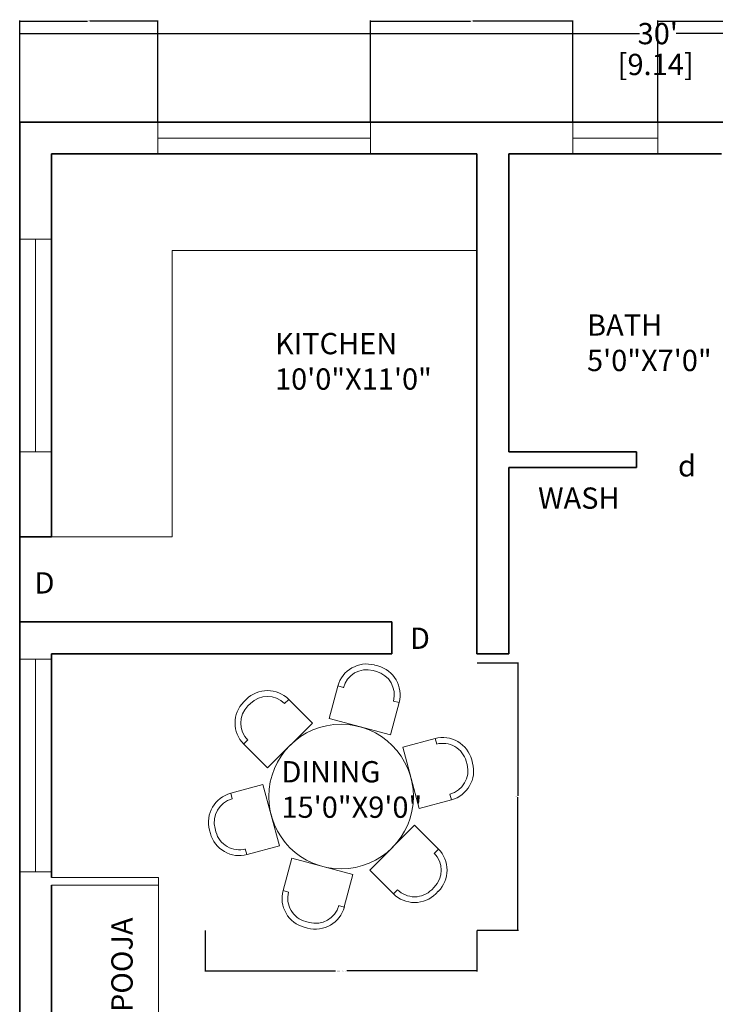
# Model space of a CAD drawing. Units: inches. Extents: x -43 to 1296, y -568 to 542.
# Tile 12 of 14: x 824 to 1020, y -253 to 25. Entities that reach past the tile are written whole.
import ezdxf

# ---------------------------------------------------------------- set-up
doc = ezdxf.new("R2010")
doc.units = ezdxf.units.IN
doc.header["$MEASUREMENT"] = 0
for name, color, linetype, lineweight in [('A-ANNO-DIMS', 2, 'Continuous', 18), ('A-ANNO-TEXT', 7, 'Continuous', 18), ('A-AREA-IDEN', 7, 'Continuous', 18), ('A-FLOR-CASE', 9, 'Continuous', 18), ('A-FURN', 8, 'Continuous', 13), ('A-GLAZ', 6, 'Continuous', 18), ('A-WALL', 7, 'Continuous', 35)]:
    doc.layers.add(name, color=color, linetype=linetype, lineweight=lineweight)
doc.styles.get("Standard").update_dxf_attribs({"font": 'arial.ttf'})
doc.dimstyles.get("Standard").update_dxf_attribs({"dimtxt": 0.18, "dimasz": 0.18, "dimexe": 0.18, "dimexo": 0.0625, "dimgap": 0.09, "dimtad": 0, "dimtih": 1, "dimtoh": 1, "dimdec": 0, "dimzin": 0, "dimdsep": 46, "dimlunit": 3, "dimtxsty": 'Standard', "dimcen": 0.09, "dimadec": 0, "dimazin": 0, "dimtfac": 1, "dimtdec": 0, "dimtofl": 0, "dimtmove": 0, "dimatfit": 3, "dimfxl": 1, "dimtolj": 1, "dimtzin": 0, "dimarcsym": 0})

# ---------------------------------------------------------------- blocks, each defined once
blk = doc.blocks.new('*D3')
at = {"layer": 'A-ANNO-DIMS', "color": 0, "lineweight": -2, "transparency": 16777216}
for p, q in [((824.13, -3.7), (824.13, 21.38)), ((824.31, 21.2), (998.95, 21.2)), ((1183.95, 21.2), (1009.31, 21.2)), ((1184.13, -3.7), (1184.13, 21.38))]:
    blk.add_line(p, q, dxfattribs=at)
at = {"layer": 'A-ANNO-DIMS', "color": 0, "transparency": 16777216}
for points in [[(824.31, 21.23), (824.31, 21.17), (824.13, 21.2)], [(1183.95, 21.23), (1183.95, 21.17), (1184.13, 21.2)]]:
    blk.add_solid(points, dxfattribs=at)
at = {"layer": 'Defpoints', "color": 0, "transparency": 16777216}
for p in [(1184.13, 21.2), (824.13, -3.76), (1184.13, -3.76)]:
    blk.add_point(p, dxfattribs=at)
at = {"layer": 'A-ANNO-DIMS', "color": 0, "transparency": 16777216, "insert": (1004.13, 21.2), "char_height": 6, "attachment_point": 5}
blk.add_mtext("\\A1;30'", dxfattribs=at)
blk = doc.blocks.new('TABLE-ROUND-6-SEAT')
for p, q in [((47.37, 72.71), (46.43, 72.96)), ((47.79, 74.28), (46.85, 74.53)), ((36.48, 68.55), (34.04, 59.43)), ((38.14, 68.18), (36.5, 68.62)), ((10.67, 64.84), (9.98, 64.15)), ((21.48, 63.69), (22.64, 64.84)), ((22.64, 64.84), (29.31, 58.16)), ((53.78, 63.91), (51.33, 54.8)), ((52.2, 64.34), (53.78, 63.91)), ((11.82, 63.69), (11.13, 63)), ((51.33, 54.8), (34.04, 59.43)), ((29.31, 58.16), (16.65, 45.5)), ((11.13, 53.43), (9.93, 52.23)), ((63.91, 53.78), (54.8, 51.33)), ((64.42, 52.15), (63.98, 53.79)), ((9.98, 52.18), (16.65, 45.5)), ((59.43, 34.04), (54.8, 51.33)), ((72.96, 46.43), (72.71, 47.37)), ((74.53, 46.85), (74.28, 47.79)), ((6.27, 38.33), (15.38, 40.77)), ((15.38, 40.77), (20.02, 23.48)), ((6.69, 36.76), (6.27, 38.33)), ((68.55, 36.49), (59.43, 34.04)), ((68.13, 38.06), (68.55, 36.49)), ((0.28, 27.97), (0.54, 27.02)), ((1.86, 28.39), (2.11, 27.44)), ((45.5, 16.65), (58.16, 29.31)), ((64.84, 22.64), (58.16, 29.31)), ((10.39, 22.66), (10.83, 21.02)), ((10.9, 21.04), (20.02, 23.48)), ((63.69, 21.38), (64.89, 22.58)), ((21.04, 10.9), (23.48, 20.02)), ((23.48, 20.02), (40.77, 15.38)), ((38.33, 6.27), (40.77, 15.38)), ((52.18, 9.98), (45.5, 16.65)), ((53.33, 11.13), (52.18, 9.98)), ((62.99, 11.13), (63.69, 11.82)), ((22.61, 10.48), (21.04, 10.9)), ((64.15, 9.98), (64.84, 10.67)), ((36.67, 6.64), (38.31, 6.2)), ((27.02, 0.54), (27.97, 0.28)), ((27.44, 2.11), (28.39, 1.86))]:
    blk.add_line(p, q)
blk.add_circle((37.41, 37.41), 20.4)
for centre, radius, start, end in [((44.66, 66.36), 8.46, 75, 165), ((44.66, 66.36), 6.83, 75, 165), ((45.6, 66.1), 6.83, 345, 75), ((45.6, 66.1), 8.46, 345, 75), ((16.65, 58.85), 8.46, 45, 135), ((15.96, 58.16), 8.46, 135, 225), ((16.65, 58.85), 6.83, 45, 135), ((15.96, 58.16), 6.83, 135, 225), ((66.1, 45.6), 8.46, 15, 105), ((66.1, 45.6), 6.83, 15, 105), ((66.36, 44.66), 6.83, 285, 15), ((66.36, 44.66), 8.46, 285, 15), ((8.46, 30.16), 8.46, 105, 195), ((8.46, 30.16), 6.83, 105, 195), ((8.71, 29.21), 8.46, 195, 285), ((8.71, 29.21), 6.83, 195, 285), ((58.85, 16.65), 8.46, 315, 45), ((58.85, 16.65), 6.83, 315, 45), ((58.16, 15.96), 6.83, 225, 315), ((29.21, 8.71), 8.46, 165, 255), ((29.21, 8.71), 6.83, 165, 255), ((58.16, 15.96), 8.46, 225, 315), ((30.16, 8.46), 8.46, 255, 345), ((30.16, 8.46), 6.83, 255, 345)]:
    blk.add_arc(centre, radius, start, end)
blk = doc.blocks.new('WIN-60x9')
for p, q in [((0, 60), (0, 0)), ((9, 60), (0, 60)), ((4.5, 60), (4.5, 0)), ((9, 0), (9, 60)), ((0, 0), (9, 0))]:
    blk.add_line(p, q)
blk = doc.blocks.new('VENT-24x9')
for p, q in [((0, 0), (0, 24)), ((0, 24), (9, 24)), ((4.5, 24), (4.5, 0)), ((9, 24), (9, 0)), ((9, 0), (0, 0))]:
    blk.add_line(p, q)
blk = doc.blocks.new('COUNTER-KITCHEN-L')
for p, q in [((34.04, 0), (34.04, 80.76)), ((34.04, 80.76), (120, 80.76)), ((0, 0), (34.04, 0))]:
    blk.add_line(p, q)
blk = doc.blocks.new('*D44')
at = {"layer": 'A-ANNO-DIMS', "color": 0, "lineweight": -2, "transparency": 16777216}
for p, q in [((876.46, -231.84), (876.46, -243.46)), ((953.12, -231.84), (953.12, -243.46)), ((876.64, -243.28), (913.19, -243.28)), ((952.94, -243.28), (916.39, -243.28))]:
    blk.add_line(p, q, dxfattribs=at)
at = {"layer": 'A-ANNO-DIMS', "color": 0, "transparency": 16777216}
for points in [[(876.64, -243.25), (876.64, -243.31), (876.46, -243.28)], [(952.94, -243.25), (952.94, -243.31), (953.12, -243.28)]]:
    blk.add_solid(points, dxfattribs=at)
at = {"layer": 'Defpoints', "color": 0, "transparency": 16777216}
for p in [(876.46, -231.78), (953.12, -231.78), (953.12, -243.28)]:
    blk.add_point(p, dxfattribs=at)
at = {"layer": 'A-ANNO-DIMS', "color": 0, "transparency": 16777216, "insert": (914.79, -243.28), "char_height": 0.18, "attachment_point": 5}
blk.add_mtext('\\A1;DINING SET 6\'-4 1/2" TYP.', dxfattribs=at)
blk = doc.blocks.new('*D45')
at = {"layer": 'A-ANNO-DIMS', "color": 0, "lineweight": -2, "transparency": 16777216}
for p, q in [((953.18, -156.37), (964.8, -156.37)), ((964.62, -156.55), (964.62, -193.89)), ((964.62, -231.6), (964.62, -194.26)), ((953.18, -231.78), (964.8, -231.78))]:
    blk.add_line(p, q, dxfattribs=at)
at = {"layer": 'A-ANNO-DIMS', "color": 0, "transparency": 16777216}
for points in [[(964.59, -156.55), (964.65, -156.55), (964.62, -156.37)], [(964.59, -231.6), (964.65, -231.6), (964.62, -231.78)]]:
    blk.add_solid(points, dxfattribs=at)
at = {"layer": 'Defpoints', "color": 0, "transparency": 16777216}
for p in [(953.12, -156.37), (964.62, -156.37), (953.12, -231.78)]:
    blk.add_point(p, dxfattribs=at)
at = {"layer": 'A-ANNO-DIMS', "color": 0, "transparency": 16777216, "insert": (964.62, -194.07), "char_height": 0.18, "attachment_point": 5}
blk.add_mtext('\\A1;6\'-3 1/2" TYP.', dxfattribs=at)
blk = doc.blocks.new('*D80')
at = {"layer": 'A-ANNO-DIMS', "color": 0, "lineweight": -2, "transparency": 16777216}
for p, q in [((824.13, -3.7), (824.13, 24.92)), ((824.31, 24.74), (843.3, 24.74)), ((862.95, 24.74), (843.96, 24.74)), ((863.13, -3.7), (863.13, 24.92))]:
    blk.add_line(p, q, dxfattribs=at)
at = {"layer": 'A-ANNO-DIMS', "color": 0, "transparency": 16777216}
for points in [[(824.31, 24.77), (824.31, 24.71), (824.13, 24.74)], [(862.95, 24.77), (862.95, 24.71), (863.13, 24.74)]]:
    blk.add_solid(points, dxfattribs=at)
at = {"layer": 'Defpoints', "color": 0, "transparency": 16777216}
for p in [(863.13, 24.74), (824.13, -3.76), (863.13, -3.76)]:
    blk.add_point(p, dxfattribs=at)
at = {"layer": 'A-ANNO-DIMS', "color": 0, "transparency": 16777216, "insert": (843.63, 24.74), "char_height": 0.18, "attachment_point": 5}
blk.add_mtext('\\A1;3\'-3"', dxfattribs=at)
blk = doc.blocks.new('*D81')
at = {"layer": 'A-ANNO-DIMS', "color": 0, "lineweight": -2, "transparency": 16777216}
for p, q in [((923.13, -3.7), (923.13, 24.92)), ((923.31, 24.74), (951.3, 24.74)), ((979.95, 24.74), (951.96, 24.74)), ((980.13, -3.7), (980.13, 24.92))]:
    blk.add_line(p, q, dxfattribs=at)
at = {"layer": 'A-ANNO-DIMS', "color": 0, "transparency": 16777216}
for points in [[(923.31, 24.77), (923.31, 24.71), (923.13, 24.74)], [(979.95, 24.77), (979.95, 24.71), (980.13, 24.74)]]:
    blk.add_solid(points, dxfattribs=at)
at = {"layer": 'Defpoints', "color": 0, "transparency": 16777216}
for p in [(980.13, 24.74), (923.13, -3.76), (980.13, -3.76)]:
    blk.add_point(p, dxfattribs=at)
at = {"layer": 'A-ANNO-DIMS', "color": 0, "transparency": 16777216, "insert": (951.63, 24.74), "char_height": 0.18, "attachment_point": 5}
blk.add_mtext('\\A1;4\'-9"', dxfattribs=at)
blk = doc.blocks.new('*D82')
at = {"layer": 'A-ANNO-DIMS', "color": 0, "lineweight": -2, "transparency": 16777216}
for p, q in [((1004.13, -3.7), (1004.13, 24.92)), ((1004.31, 24.74), (1038.3, 24.74)), ((1072.95, 24.74), (1038.96, 24.74)), ((1073.13, -3.7), (1073.13, 24.92))]:
    blk.add_line(p, q, dxfattribs=at)
at = {"layer": 'A-ANNO-DIMS', "color": 0, "transparency": 16777216}
for points in [[(1004.31, 24.77), (1004.31, 24.71), (1004.13, 24.74)], [(1072.95, 24.77), (1072.95, 24.71), (1073.13, 24.74)]]:
    blk.add_solid(points, dxfattribs=at)
at = {"layer": 'Defpoints', "color": 0, "transparency": 16777216}
for p in [(1073.13, 24.74), (1004.13, -3.76), (1073.13, -3.76)]:
    blk.add_point(p, dxfattribs=at)
at = {"layer": 'A-ANNO-DIMS', "color": 0, "transparency": 16777216, "insert": (1038.63, 24.74), "char_height": 0.18, "attachment_point": 5}
blk.add_mtext('\\A1;5\'-9"', dxfattribs=at)

msp = doc.modelspace()

# ---------------------------------------------------------------- linework, layer by layer
at = {"layer": 'A-FLOR-CASE'}
for p, q in [((833.13, -216.91), (863.31, -216.91)), ((863.31, -219.05), (833.13, -219.05)), ((863.31, -216.91), (863.31, -219.05)), ((863.31, -261.76), (863.31, -219.05))]:
    msp.add_line(p, q, dxfattribs=at)
at = {"layer": 'A-WALL'}
for p, q in [((824.13, -3.76), (824.13, -483.76)), ((824.13, -3.76), (1184.13, -3.76)), ((833.13, -12.76), (833.13, -120.76)), ((833.13, -12.76), (953.13, -12.76)), ((953.13, -12.76), (953.13, -153.76)), ((962.13, -12.76), (962.13, -96.76)), ((962.13, -12.76), (1022.13, -12.76)), ((962.13, -96.76), (998.13, -96.76)), ((998.13, -101.26), (998.13, -96.76)), ((962.13, -101.26), (962.13, -153.76)), ((962.13, -101.26), (998.13, -101.26)), ((833.13, -120.76), (824.13, -120.76)), ((833.13, -144.76), (824.13, -144.76)), ((833.13, -144.76), (929.13, -144.76)), ((929.13, -153.76), (929.13, -144.76)), ((833.13, -153.76), (833.13, -216.91)), ((833.13, -153.76), (929.13, -153.76)), ((953.13, -153.76), (962.13, -153.76)), ((833.13, -219.05), (833.13, -261.76))]:
    msp.add_line(p, q, dxfattribs=at)

# ---------------------------------------------------------------- block references
at = {"layer": 'A-FLOR-CASE'}
msp.add_blockref('COUNTER-KITCHEN-L', (833.13, -120.76), dxfattribs=at)
at = {"layer": 'A-FURN'}
msp.add_blockref('TABLE-ROUND-6-SEAT', (877.38, -231.48), dxfattribs=at)
at = {"layer": 'A-GLAZ'}
for name, p, rotation in [('WIN-60x9', (863.13, -3.76), 270.0000000000002), ('VENT-24x9', (980.13, -3.76), 269.999999999999)]:
    msp.add_blockref(name, p, dxfattribs=dict(at, rotation=rotation))
for p in [(824.13, -96.76), (824.13, -215.34)]:
    msp.add_blockref('WIN-60x9', p, dxfattribs=at)

# ---------------------------------------------------------------- texts
at = {"layer": 'A-ANNO-DIMS', "insert": (992.82, 15.5), "char_height": 6, "attachment_point": 1}
msp.add_mtext_dynamic_manual_height_columns('[9.14]', width=0.2388, gutter_width=1, heights=[0], dxfattribs=at)
at = {"layer": 'A-ANNO-TEXT', "char_height": 6, "attachment_point": 1}
for s, insert in [('d', (1009.83, -97.76)), ('D', (934.22, -146.41))]:
    msp.add_mtext(s, dxfattribs=dict(at, insert=insert))
at = {"layer": 'A-ANNO-TEXT', "insert": (828.32, -130.78), "char_height": 6, "attachment_point": 1}
msp.add_mtext_dynamic_manual_height_columns('D', width=0.5519, gutter_width=1, heights=[0], dxfattribs=at)
at = {"layer": 'A-AREA-IDEN', "char_height": 6, "attachment_point": 1}
for s, insert in [('BATH\\P5\'0"X7\'0"', (984.17, -58.02)), ('KITCHEN\\P10\'0"X11\'0"', (896.14, -63.26)), ('WASH', (970.37, -106.86)), ('DINING\\P15\'0"X9\'0"', (897.98, -184.07))]:
    msp.add_mtext(s, dxfattribs=dict(at, insert=insert))
at = {"layer": 'A-AREA-IDEN', "insert": (849.99, -254.87), "char_height": 6, "attachment_point": 1, "rotation": 90}
msp.add_mtext('POOJA', dxfattribs=at)

# ---------------------------------------------------------------- dimensions: what is measured, and where the dimension line sits
at = {"layer": 'A-ANNO-DIMS'}
for base, p1, p2, override, picture, middle in [((1184.13, 21.2), (824.13, -3.76), (1184.13, -3.76), {"dimtxt": 6, "dimclrd": 0, "dimclre": 0, "dimclrt": 0}, '*D3', (1004.13, 21.2)), ((863.13, 24.74), (824.13, -3.76), (863.13, -3.76), {"dimdec": 1, "dimlfac": 1, "dimrnd": 0, "dimzin": 1, "dimdsep": 46, "dimlunit": 4, "dimfrac": 2}, '*D80', (843.63, 24.74)), ((980.13, 24.74), (923.13, -3.76), (980.13, -3.76), {"dimdec": 1, "dimlfac": 1, "dimrnd": 0, "dimzin": 1, "dimdsep": 46, "dimlunit": 4, "dimfrac": 2}, '*D81', (951.63, 24.74)), ((1073.13, 24.74), (1004.13, -3.76), (1073.13, -3.76), {"dimdec": 1, "dimlfac": 1, "dimrnd": 0, "dimzin": 1, "dimdsep": 46, "dimlunit": 4, "dimfrac": 2}, '*D82', (1038.63, 24.74))]:
    dim = msp.add_linear_dim(base=base, p1=p1, p2=p2, dimstyle='Standard', override=override, dxfattribs=at)
    dim.commit()
    dim.dimension.update_dxf_attribs({"geometry": picture, "text_midpoint": middle})
dim = msp.add_linear_dim(base=(964.62, -156.37), p1=(953.12, -231.78), p2=(953.12, -156.37), angle=90, text='<> TYP.', dimstyle='Standard', override={"dimdec": 1, "dimlfac": 1, "dimrnd": 0, "dimzin": 1, "dimdsep": 46, "dimlunit": 4, "dimfrac": 2}, dxfattribs=at)
dim.commit()
dim.dimension.update_dxf_attribs({"geometry": '*D45', "text_midpoint": (964.62, -194.07)})
dim = msp.add_linear_dim(base=(953.12, -243.28), p1=(876.46, -231.78), p2=(953.12, -231.78), text='DINING SET <> TYP.', dimstyle='Standard', override={"dimdec": 1, "dimlfac": 1, "dimrnd": 0, "dimzin": 1, "dimdsep": 46, "dimlunit": 4, "dimfrac": 2}, dxfattribs=at)
dim.commit()
dim.dimension.update_dxf_attribs({"geometry": '*D44', "text_midpoint": (914.79, -243.28)})

doc.saveas('drawing.dxf')
